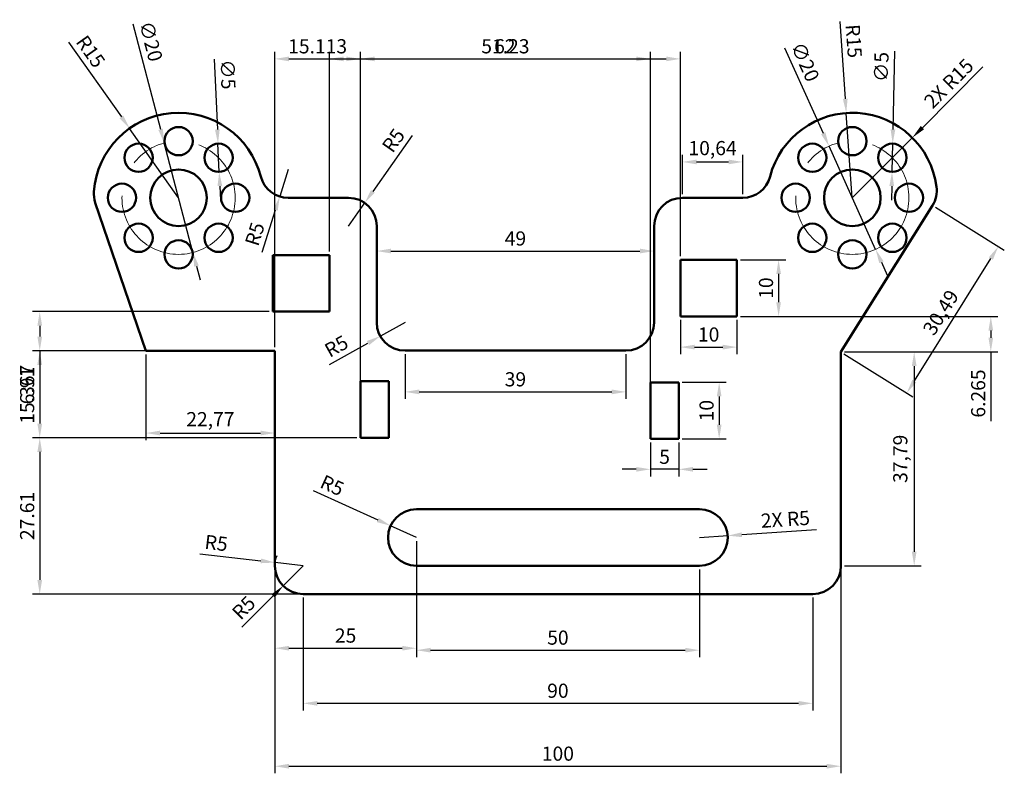
# Model space of a CAD drawing. Units: millimetres. Extents: x 1154 to 1562, y 1225 to 1481.
# Tile 3 of 4: x 1388 to 1562, y 1225 to 1358. Entities that reach past the tile are written whole.
import ezdxf

# ---------------------------------------------------------------- set-up
doc = ezdxf.new("R2010")
doc.units = ezdxf.units.MM
doc.linetypes.add('CENTER', pattern=[50.8, 31.75, -6.35, 6.35, -6.35])
for name, color, linetype, lineweight in [('M-CNTR', 1, 'CENTER', 18), ('M-DIMS', 2, 'Continuous', 25), ('M-OUTL', 7, 'Continuous', 50)]:
    doc.layers.add(name, color=color, linetype=linetype, lineweight=lineweight)
doc.styles.get("Standard").update_dxf_attribs({"font": 'arial.ttf'})
doc.dimstyles.new('ISO-25', dxfattribs={"dimtxt": 2.5, "dimasz": 2.5, "dimexe": 1.25, "dimexo": 0.625, "dimtad": 1, "dimtxsty": 'Standard', "dimcen": 2.5, "dimadec": 0, "dimazin": 0, "dimtfac": 1, "dimtmove": 0, "dimatfit": 3, "dimfxl": 1, "dimarcsym": 0})

# ---------------------------------------------------------------- blocks, each defined once
blk = doc.blocks.new('*U3')
blk.add_circle((0, 0), 2.5)
blk = doc.blocks.new('*U4')
at = {"layer": 'M-OUTL', "color": 0, "linetype": 'ByBlock', "lineweight": -2, "transparency": 16777216}
blk.add_blockref('*U3', (1535.28, 1336.67), dxfattribs=at)
for p, rotation in [((1528.21, 1333.74), 45.00000000000001), ((1542.35, 1333.74), 315), ((1525.28, 1326.67), 90), ((1545.28, 1326.67), 270), ((1528.21, 1319.6), 135), ((1542.35, 1319.6), 225), ((1535.28, 1316.67), 180)]:
    blk.add_blockref('*U3', p, dxfattribs=dict(at, rotation=rotation))
blk = doc.blocks.new('*U5')
blk.add_circle((0, 0), 2.5)
blk = doc.blocks.new('*U6')
at = {"layer": 'M-OUTL', "color": 0, "linetype": 'ByBlock', "lineweight": -2, "transparency": 16777216}
blk.add_blockref('*U5', (1416.28, 1336.67), dxfattribs=at)
for p, rotation in [((1409.21, 1333.74), 45.00000000000001), ((1423.35, 1333.74), 315), ((1406.28, 1326.67), 90), ((1426.28, 1326.67), 270), ((1409.21, 1319.6), 135), ((1423.35, 1319.6), 225), ((1416.28, 1316.67), 180)]:
    blk.add_blockref('*U5', p, dxfattribs=dict(at, rotation=rotation))
blk = doc.blocks.new('*D32')
at = {"layer": 'Defpoints', "color": 0, "transparency": 16777216}
for p in [(1407.63, 1338.92), (1416.28, 1326.67)]:
    blk.add_point(p, dxfattribs=at)
at = {"layer": 'M-DIMS', "color": 0, "lineweight": -2, "transparency": 16777216}
for p, q in [((1396.85, 1354.17), (1406.18, 1340.97)), ((1416.28, 1326.67), (1407.63, 1338.92))]:
    blk.add_line(p, q, dxfattribs=at)
at = {"layer": 'M-DIMS', "color": 0, "transparency": 16777216}
blk.add_solid([(1406.52, 1341.21), (1405.84, 1340.72), (1407.63, 1338.92)], dxfattribs=at)
at = {"layer": 'M-DIMS', "color": 0, "transparency": 16777216, "insert": (1400.49, 1352.31), "char_height": 2.5, "attachment_point": 5, "rotation": 305.247}
blk.add_mtext('R15', dxfattribs=at)
blk = doc.blocks.new('*D33')
at = {"layer": 'Defpoints', "color": 0, "transparency": 16777216}
for p in [(1413.74, 1336.35), (1418.82, 1317)]:
    blk.add_point(p, dxfattribs=at)
at = {"layer": 'M-DIMS', "color": 0, "lineweight": -2, "transparency": 16777216}
for p, q in [((1408.23, 1357.37), (1413.11, 1338.76)), ((1418.82, 1317), (1413.74, 1336.35)), ((1419.45, 1314.58), (1420.09, 1312.16))]:
    blk.add_line(p, q, dxfattribs=at)
at = {"layer": 'M-DIMS', "color": 0, "transparency": 16777216}
for points in [[(1413.51, 1338.87), (1412.71, 1338.66), (1413.74, 1336.35)], [(1419.86, 1314.69), (1419.05, 1314.48), (1418.82, 1317)]]:
    blk.add_solid(points, dxfattribs=at)
at = {"layer": 'M-DIMS', "color": 0, "transparency": 16777216, "insert": (1411.09, 1354.22), "char_height": 2.5, "attachment_point": 5, "rotation": 284.7028}
blk.add_mtext('∅20', dxfattribs=at)
blk = doc.blocks.new('*D34')
at = {"layer": 'Defpoints', "color": 0, "transparency": 16777216}
for p in [(1423.24, 1336.24), (1423.46, 1331.25)]:
    blk.add_point(p, dxfattribs=at)
at = {"layer": 'M-DIMS', "color": 0, "lineweight": -2, "transparency": 16777216}
for p, q in [((1422.58, 1351.16), (1423.13, 1338.74)), ((1423.46, 1331.25), (1423.24, 1336.24)), ((1423.57, 1328.75), (1423.69, 1326.25))]:
    blk.add_line(p, q, dxfattribs=at)
at = {"layer": 'M-DIMS', "color": 0, "transparency": 16777216}
for points in [[(1423.55, 1338.76), (1422.71, 1338.72), (1423.24, 1336.24)], [(1423.99, 1328.77), (1423.16, 1328.73), (1423.46, 1331.25)]]:
    blk.add_solid(points, dxfattribs=at)
at = {"layer": 'M-DIMS', "color": 0, "transparency": 16777216, "insert": (1424.67, 1348.44), "char_height": 2.5, "attachment_point": 5, "rotation": 272.5448}
blk.add_mtext('∅5', dxfattribs=at)
blk = doc.blocks.new('*D35')
at = {"layer": 'Defpoints', "color": 0, "transparency": 16777216}
for p in [(1531.17, 1335.79), (1539.4, 1317.56)]:
    blk.add_point(p, dxfattribs=at)
at = {"layer": 'M-DIMS', "color": 0, "lineweight": -2, "transparency": 16777216}
for p, q in [((1523.32, 1353.17), (1530.14, 1338.07)), ((1539.4, 1317.56), (1531.17, 1335.79)), ((1540.43, 1315.28), (1541.46, 1313))]:
    blk.add_line(p, q, dxfattribs=at)
at = {"layer": 'M-DIMS', "color": 0, "transparency": 16777216}
for points in [[(1530.52, 1338.24), (1529.76, 1337.89), (1531.17, 1335.79)], [(1540.81, 1315.45), (1540.05, 1315.11), (1539.4, 1317.56)]]:
    blk.add_solid(points, dxfattribs=at)
at = {"layer": 'M-DIMS', "color": 0, "transparency": 16777216, "insert": (1526.67, 1350.54), "char_height": 2.5, "attachment_point": 5, "rotation": 294.3018}
blk.add_mtext('∅20', dxfattribs=at)
blk = doc.blocks.new('*D36')
at = {"layer": 'Defpoints', "color": 0, "transparency": 16777216}
for p in [(1542.41, 1336.24), (1542.3, 1331.25)]:
    blk.add_point(p, dxfattribs=at)
at = {"layer": 'M-DIMS', "color": 0, "lineweight": -2, "transparency": 16777216}
for p, q in [((1542.75, 1352.55), (1542.46, 1338.74)), ((1542.3, 1331.25), (1542.41, 1336.24)), ((1542.25, 1328.75), (1542.19, 1326.25))]:
    blk.add_line(p, q, dxfattribs=at)
at = {"layer": 'M-DIMS', "color": 0, "transparency": 16777216}
for points in [[(1542.04, 1338.75), (1542.88, 1338.73), (1542.41, 1336.24)], [(1541.83, 1328.75), (1542.66, 1328.74), (1542.3, 1331.25)]]:
    blk.add_solid(points, dxfattribs=at)
at = {"layer": 'M-DIMS', "color": 0, "transparency": 16777216, "insert": (1540.72, 1349.77), "char_height": 2.5, "attachment_point": 5, "rotation": 88.7888}
blk.add_mtext('∅5', dxfattribs=at)
blk = doc.blocks.new('*D37')
at = {"layer": 'Defpoints', "color": 0, "transparency": 16777216}
for p in [(1534.21, 1341.64), (1535.28, 1326.67)]:
    blk.add_point(p, dxfattribs=at)
at = {"layer": 'M-DIMS', "color": 0, "lineweight": -2, "transparency": 16777216}
for p, q in [((1533.06, 1357.8), (1534.04, 1344.13)), ((1535.28, 1326.67), (1534.21, 1341.64))]:
    blk.add_line(p, q, dxfattribs=at)
at = {"layer": 'M-DIMS', "color": 0, "transparency": 16777216}
blk.add_solid([(1534.45, 1344.16), (1533.62, 1344.1), (1534.21, 1341.64)], dxfattribs=at)
at = {"layer": 'M-DIMS', "color": 0, "transparency": 16777216, "insert": (1535.22, 1354.32), "char_height": 2.5, "attachment_point": 5, "rotation": 274.0804}
blk.add_mtext('R15', dxfattribs=at)
blk = doc.blocks.new('*D38')
at = {"layer": 'Defpoints', "color": 0, "transparency": 16777216}
for p in [(1504.91, 1305.72), (1514.91, 1305.72), (1514.91, 1300.3)]:
    blk.add_point(p, dxfattribs=at)
at = {"layer": 'M-DIMS', "color": 0, "lineweight": -2, "transparency": 16777216}
for p, q in [((1504.91, 1305.1), (1504.91, 1299.05)), ((1514.91, 1305.1), (1514.91, 1299.05)), ((1507.41, 1300.3), (1512.41, 1300.3))]:
    blk.add_line(p, q, dxfattribs=at)
at = {"layer": 'M-DIMS', "color": 0, "transparency": 16777216}
for points in [[(1507.41, 1300.72), (1507.41, 1299.88), (1504.91, 1300.3)], [(1512.41, 1300.72), (1512.41, 1299.88), (1514.91, 1300.3)]]:
    blk.add_solid(points, dxfattribs=at)
at = {"layer": 'M-DIMS', "color": 0, "transparency": 16777216, "insert": (1509.91, 1302.2), "char_height": 2.5, "attachment_point": 5}
blk.add_mtext('10', dxfattribs=at)
blk = doc.blocks.new('*D39')
at = {"layer": 'Defpoints', "color": 0, "transparency": 16777216}
for p in [(1514.91, 1315.72), (1514.91, 1305.72), (1522.26, 1305.72)]:
    blk.add_point(p, dxfattribs=at)
at = {"layer": 'M-DIMS', "color": 0, "lineweight": -2, "transparency": 16777216}
for p, q in [((1515.54, 1315.72), (1523.51, 1315.72)), ((1522.26, 1313.22), (1522.26, 1308.22)), ((1515.54, 1305.72), (1523.51, 1305.72))]:
    blk.add_line(p, q, dxfattribs=at)
at = {"layer": 'M-DIMS', "color": 0, "transparency": 16777216}
for points in [[(1521.85, 1313.22), (1522.68, 1313.22), (1522.26, 1315.72)], [(1521.85, 1308.22), (1522.68, 1308.22), (1522.26, 1305.72)]]:
    blk.add_solid(points, dxfattribs=at)
at = {"layer": 'M-DIMS', "color": 0, "transparency": 16777216, "insert": (1520.36, 1310.72), "char_height": 2.5, "attachment_point": 5, "rotation": 90}
blk.add_mtext('10', dxfattribs=at)
blk = doc.blocks.new('*D40')
at = {"layer": 'Defpoints', "color": 0, "transparency": 16777216}
for p in [(1504.62, 1294.08), (1504.62, 1284.08), (1511.76, 1284.08)]:
    blk.add_point(p, dxfattribs=at)
at = {"layer": 'M-DIMS', "color": 0, "lineweight": -2, "transparency": 16777216}
for p, q in [((1505.25, 1294.08), (1513.01, 1294.08)), ((1511.76, 1291.58), (1511.76, 1286.58)), ((1505.25, 1284.08), (1513.01, 1284.08))]:
    blk.add_line(p, q, dxfattribs=at)
at = {"layer": 'M-DIMS', "color": 0, "transparency": 16777216}
for points in [[(1511.35, 1291.58), (1512.18, 1291.58), (1511.76, 1294.08)], [(1511.35, 1286.58), (1512.18, 1286.58), (1511.76, 1284.08)]]:
    blk.add_solid(points, dxfattribs=at)
at = {"layer": 'M-DIMS', "color": 0, "transparency": 16777216, "insert": (1509.86, 1289.08), "char_height": 2.5, "attachment_point": 5, "rotation": 90}
blk.add_mtext('10', dxfattribs=at)
blk = doc.blocks.new('*D41')
at = {"layer": 'Defpoints', "color": 0, "transparency": 16777216}
for p in [(1499.62, 1284.08), (1504.62, 1284.08), (1499.62, 1278.72)]:
    blk.add_point(p, dxfattribs=at)
at = {"layer": 'M-DIMS', "color": 0, "lineweight": -2, "transparency": 16777216}
for p, q in [((1499.62, 1283.45), (1499.62, 1277.47)), ((1504.62, 1283.45), (1504.62, 1277.47)), ((1497.12, 1278.72), (1494.62, 1278.72)), ((1504.62, 1278.72), (1499.62, 1278.72)), ((1507.12, 1278.72), (1509.62, 1278.72))]:
    blk.add_line(p, q, dxfattribs=at)
at = {"layer": 'M-DIMS', "color": 0, "transparency": 16777216}
for points in [[(1497.12, 1279.13), (1497.12, 1278.3), (1499.62, 1278.72)], [(1507.12, 1279.13), (1507.12, 1278.3), (1504.62, 1278.72)]]:
    blk.add_solid(points, dxfattribs=at)
at = {"layer": 'M-DIMS', "color": 0, "transparency": 16777216, "insert": (1502.12, 1280.61), "char_height": 2.5, "attachment_point": 5}
blk.add_mtext('5', dxfattribs=at)
blk = doc.blocks.new('*D42')
at = {"layer": 'Defpoints', "color": 0, "transparency": 16777216}
for p in [(1458.28, 1261.67), (1508.28, 1261.67), (1508.28, 1246.77)]:
    blk.add_point(p, dxfattribs=at)
at = {"layer": 'M-DIMS', "color": 0, "lineweight": -2, "transparency": 16777216}
for p, q in [((1458.28, 1261.05), (1458.28, 1245.52)), ((1508.28, 1261.05), (1508.28, 1245.52)), ((1460.78, 1246.77), (1505.78, 1246.77))]:
    blk.add_line(p, q, dxfattribs=at)
at = {"layer": 'M-DIMS', "color": 0, "transparency": 16777216}
for points in [[(1460.78, 1247.19), (1460.78, 1246.36), (1458.28, 1246.77)], [(1505.78, 1247.19), (1505.78, 1246.36), (1508.28, 1246.77)]]:
    blk.add_solid(points, dxfattribs=at)
at = {"layer": 'M-DIMS', "color": 0, "transparency": 16777216, "insert": (1483.28, 1248.67), "char_height": 2.5, "attachment_point": 5}
blk.add_mtext('50', dxfattribs=at)
blk = doc.blocks.new('*D43')
at = {"layer": 'Defpoints', "color": 0, "transparency": 16777216}
for p in [(1410.51, 1299.65), (1433.28, 1299.65), (1433.28, 1285.12)]:
    blk.add_point(p, dxfattribs=at)
at = {"layer": 'M-DIMS', "color": 0, "lineweight": -2, "transparency": 16777216}
for p, q in [((1410.51, 1299.02), (1410.51, 1283.87)), ((1433.28, 1299.02), (1433.28, 1283.87)), ((1413.01, 1285.12), (1430.78, 1285.12))]:
    blk.add_line(p, q, dxfattribs=at)
at = {"layer": 'M-DIMS', "color": 0, "transparency": 16777216}
for points in [[(1413.01, 1285.54), (1413.01, 1284.71), (1410.51, 1285.12)], [(1430.78, 1285.54), (1430.78, 1284.71), (1433.28, 1285.12)]]:
    blk.add_solid(points, dxfattribs=at)
at = {"layer": 'M-DIMS', "color": 0, "transparency": 16777216, "insert": (1421.9, 1287.25), "char_height": 2.5, "attachment_point": 5}
blk.add_mtext('22,77', dxfattribs=at)
blk = doc.blocks.new('*D44')
at = {"layer": 'Defpoints', "color": 0, "transparency": 16777216}
for p in [(1453.73, 1268.74), (1458.28, 1266.67)]:
    blk.add_point(p, dxfattribs=at)
at = {"layer": 'M-DIMS', "color": 0, "lineweight": -2, "transparency": 16777216}
for p, q in [((1440.08, 1274.95), (1451.45, 1269.78)), ((1458.28, 1266.67), (1453.73, 1268.74))]:
    blk.add_line(p, q, dxfattribs=at)
at = {"layer": 'M-DIMS', "color": 0, "transparency": 16777216}
blk.add_solid([(1451.63, 1270.16), (1451.28, 1269.4), (1453.73, 1268.74)], dxfattribs=at)
at = {"layer": 'M-DIMS', "color": 0, "transparency": 16777216, "insert": (1443.28, 1275.58), "char_height": 2.5, "attachment_point": 5, "rotation": 335.543}
blk.add_mtext('R5', dxfattribs=at)
blk = doc.blocks.new('*D45')
at = {"layer": 'Defpoints', "color": 0, "transparency": 16777216}
for p in [(1433.32, 1262.25), (1438.28, 1261.67)]:
    blk.add_point(p, dxfattribs=at)
at = {"layer": 'M-DIMS', "color": 0, "lineweight": -2, "transparency": 16777216}
for p, q in [((1420.05, 1263.8), (1430.83, 1262.54)), ((1438.28, 1261.67), (1433.32, 1262.25))]:
    blk.add_line(p, q, dxfattribs=at)
blk.add_arc((1438.28, 1261.67), 5, 159.0215, 180, dxfattribs=at)
at = {"layer": 'M-DIMS', "color": 0, "transparency": 16777216}
blk.add_solid([(1430.88, 1262.96), (1430.78, 1262.13), (1433.32, 1262.25)], dxfattribs=at)
at = {"layer": 'M-DIMS', "color": 0, "transparency": 16777216, "insert": (1422.9, 1265.38), "char_height": 2.5, "attachment_point": 5, "rotation": 353.3454}
blk.add_mtext('R5', dxfattribs=at)
blk = doc.blocks.new('*D46')
at = {"layer": 'Defpoints', "color": 0, "transparency": 16777216}
for p in [(1449.16, 1325.76), (1446.28, 1321.67)]:
    blk.add_point(p, dxfattribs=at)
at = {"layer": 'M-DIMS', "color": 0, "lineweight": -2, "transparency": 16777216}
for p, q in [((1457.56, 1337.69), (1450.6, 1327.8)), ((1446.28, 1321.67), (1449.16, 1325.76))]:
    blk.add_line(p, q, dxfattribs=at)
at = {"layer": 'M-DIMS', "color": 0, "transparency": 16777216}
blk.add_solid([(1450.26, 1328.04), (1450.94, 1327.57), (1449.16, 1325.76)], dxfattribs=at)
at = {"layer": 'M-DIMS', "color": 0, "transparency": 16777216, "insert": (1454.49, 1336.61), "char_height": 2.5, "attachment_point": 5, "rotation": 54.837}
blk.add_mtext('R5', dxfattribs=at)
blk = doc.blocks.new('*D47')
at = {"layer": 'Defpoints', "color": 0, "transparency": 16777216}
for p in [(1435.65, 1331.67), (1434.15, 1326.9)]:
    blk.add_point(p, dxfattribs=at)
at = {"layer": 'M-DIMS', "color": 0, "lineweight": -2, "transparency": 16777216}
for p, q in [((1435.65, 1331.67), (1434.15, 1326.9)), ((1431.07, 1317.07), (1433.41, 1324.52))]:
    blk.add_line(p, q, dxfattribs=at)
at = {"layer": 'M-DIMS', "color": 0, "transparency": 16777216}
blk.add_solid([(1433.01, 1324.64), (1433.8, 1324.39), (1434.15, 1326.9)], dxfattribs=at)
at = {"layer": 'M-DIMS', "color": 0, "transparency": 16777216, "insert": (1430.06, 1320.17), "char_height": 2.5, "attachment_point": 5, "rotation": 72.6131}
blk.add_mtext('R5', dxfattribs=at)
blk = doc.blocks.new('*D48')
at = {"layer": 'Defpoints', "color": 0, "transparency": 16777216}
for p in [(1456.28, 1304.67), (1451.92, 1302.24)]:
    blk.add_point(p, dxfattribs=at)
at = {"layer": 'M-DIMS', "color": 0, "lineweight": -2, "transparency": 16777216}
for p, q in [((1456.28, 1304.67), (1451.92, 1302.24)), ((1442.92, 1297.22), (1449.73, 1301.02))]:
    blk.add_line(p, q, dxfattribs=at)
at = {"layer": 'M-DIMS', "color": 0, "transparency": 16777216}
blk.add_solid([(1449.53, 1301.38), (1449.94, 1300.66), (1451.92, 1302.24)], dxfattribs=at)
at = {"layer": 'M-DIMS', "color": 0, "transparency": 16777216, "insert": (1444.31, 1300.17), "char_height": 2.5, "attachment_point": 5, "rotation": 29.1577}
blk.add_mtext('R5', dxfattribs=at)
blk = doc.blocks.new('*D49')
at = {"layer": 'Defpoints', "color": 0, "transparency": 16777216}
for p in [(1438.28, 1256.67), (1528.28, 1256.67), (1528.28, 1237.39)]:
    blk.add_point(p, dxfattribs=at)
at = {"layer": 'M-DIMS', "color": 0, "lineweight": -2, "transparency": 16777216}
for p, q in [((1438.28, 1256.05), (1438.28, 1236.14)), ((1528.28, 1256.05), (1528.28, 1236.14)), ((1440.78, 1237.39), (1525.78, 1237.39))]:
    blk.add_line(p, q, dxfattribs=at)
at = {"layer": 'M-DIMS', "color": 0, "transparency": 16777216}
for points in [[(1440.78, 1237.8), (1440.78, 1236.97), (1438.28, 1237.39)], [(1525.78, 1237.8), (1525.78, 1236.97), (1528.28, 1237.39)]]:
    blk.add_solid(points, dxfattribs=at)
at = {"layer": 'M-DIMS', "color": 0, "transparency": 16777216, "insert": (1483.28, 1239.29), "char_height": 2.5, "attachment_point": 5}
blk.add_mtext('90', dxfattribs=at)
blk = doc.blocks.new('*D50')
at = {"layer": 'Defpoints', "color": 0, "transparency": 16777216}
for p in [(1433.28, 1261.67), (1533.28, 1261.67), (1533.28, 1226.28)]:
    blk.add_point(p, dxfattribs=at)
at = {"layer": 'M-DIMS', "color": 0, "lineweight": -2, "transparency": 16777216}
for p, q in [((1433.28, 1261.05), (1433.28, 1225.03)), ((1533.28, 1261.05), (1533.28, 1225.03)), ((1435.78, 1226.28), (1530.78, 1226.28))]:
    blk.add_line(p, q, dxfattribs=at)
at = {"layer": 'M-DIMS', "color": 0, "transparency": 16777216}
for points in [[(1435.78, 1226.7), (1435.78, 1225.86), (1433.28, 1226.28)], [(1530.78, 1226.7), (1530.78, 1225.86), (1533.28, 1226.28)]]:
    blk.add_solid(points, dxfattribs=at)
at = {"layer": 'M-DIMS', "color": 0, "transparency": 16777216, "insert": (1483.28, 1228.18), "char_height": 2.5, "attachment_point": 5}
blk.add_mtext('100', dxfattribs=at)
blk = doc.blocks.new('*D59')
at = {"layer": 'Defpoints', "color": 0, "transparency": 16777216}
for p in [(1456.28, 1299.67), (1495.28, 1299.67), (1495.28, 1292.39)]:
    blk.add_point(p, dxfattribs=at)
at = {"layer": 'M-DIMS', "color": 0, "lineweight": -2, "transparency": 16777216}
for p, q in [((1456.28, 1299.05), (1456.28, 1291.14)), ((1495.28, 1299.05), (1495.28, 1291.14)), ((1458.78, 1292.39), (1492.78, 1292.39))]:
    blk.add_line(p, q, dxfattribs=at)
at = {"layer": 'M-DIMS', "color": 0, "transparency": 16777216}
for points in [[(1458.78, 1292.81), (1458.78, 1291.97), (1456.28, 1292.39)], [(1492.78, 1292.81), (1492.78, 1291.97), (1495.28, 1292.39)]]:
    blk.add_solid(points, dxfattribs=at)
at = {"layer": 'M-DIMS', "color": 0, "transparency": 16777216, "insert": (1475.78, 1294.29), "char_height": 2.5, "attachment_point": 5}
blk.add_mtext('39', dxfattribs=at)
blk = doc.blocks.new('*D62')
at = {"layer": 'Defpoints', "color": 0, "transparency": 16777216}
for p in [(1500.28, 1317.26), (1451.28, 1313.17), (1500.28, 1313.17)]:
    blk.add_point(p, dxfattribs=at)
at = {"layer": 'M-DIMS', "color": 0, "lineweight": -2, "transparency": 16777216}
for p, q in [((1451.28, 1313.8), (1451.28, 1318.51)), ((1500.28, 1313.8), (1500.28, 1318.51)), ((1453.78, 1317.26), (1497.78, 1317.26))]:
    blk.add_line(p, q, dxfattribs=at)
at = {"layer": 'M-DIMS', "color": 0, "transparency": 16777216}
for points in [[(1453.78, 1317.68), (1453.78, 1316.85), (1451.28, 1317.26)], [(1497.78, 1317.68), (1497.78, 1316.85), (1500.28, 1317.26)]]:
    blk.add_solid(points, dxfattribs=at)
at = {"layer": 'M-DIMS', "color": 0, "transparency": 16777216, "insert": (1475.78, 1319.16), "char_height": 2.5, "attachment_point": 5}
blk.add_mtext('49', dxfattribs=at)
blk = doc.blocks.new('*D63')
at = {"layer": 'Defpoints', "color": 0, "transparency": 16777216}
for p in [(1515.92, 1333), (1505.28, 1326.67), (1515.92, 1326.67)]:
    blk.add_point(p, dxfattribs=at)
at = {"layer": 'M-DIMS', "color": 0, "lineweight": -2, "transparency": 16777216}
for p, q in [((1505.28, 1327.3), (1505.28, 1334.25)), ((1515.92, 1327.3), (1515.92, 1334.25)), ((1507.78, 1333), (1513.42, 1333))]:
    blk.add_line(p, q, dxfattribs=at)
at = {"layer": 'M-DIMS', "color": 0, "transparency": 16777216}
for points in [[(1507.78, 1333.41), (1507.78, 1332.58), (1505.28, 1333)], [(1513.42, 1333.41), (1513.42, 1332.58), (1515.92, 1333)]]:
    blk.add_solid(points, dxfattribs=at)
at = {"layer": 'M-DIMS', "color": 0, "transparency": 16777216, "insert": (1510.6, 1335.12), "char_height": 2.5, "attachment_point": 5}
blk.add_mtext('10,64', dxfattribs=at)
blk = doc.blocks.new('*D64')
at = {"layer": 'Defpoints', "color": 0, "transparency": 16777216}
for p in [(1549.44, 1325.32), (1561.07, 1318.06), (1533.28, 1299.46)]:
    blk.add_point(p, dxfattribs=at)
at = {"layer": 'M-DIMS', "color": 0, "lineweight": -2, "transparency": 16777216}
for p, q in [((1549.97, 1324.99), (1562.13, 1317.4)), ((1546.24, 1294.32), (1559.74, 1315.94)), ((1533.81, 1299.13), (1545.97, 1291.53))]:
    blk.add_line(p, q, dxfattribs=at)
at = {"layer": 'M-DIMS', "color": 0, "transparency": 16777216}
for points in [[(1559.39, 1316.16), (1560.1, 1315.72), (1561.07, 1318.06)], [(1545.88, 1294.54), (1546.59, 1294.09), (1544.91, 1292.2)]]:
    blk.add_solid(points, dxfattribs=at)
at = {"layer": 'M-DIMS', "color": 0, "transparency": 16777216, "insert": (1551.18, 1306.25), "char_height": 2.5, "attachment_point": 5, "rotation": 58.0079}
blk.add_mtext('30,49', dxfattribs=at)
blk = doc.blocks.new('*D65')
at = {"layer": 'Defpoints', "color": 0, "transparency": 16777216}
for p in [(1533.28, 1299.46), (1533.28, 1261.67), (1546.21, 1261.67)]:
    blk.add_point(p, dxfattribs=at)
at = {"layer": 'M-DIMS', "color": 0, "lineweight": -2, "transparency": 16777216}
for p, q in [((1533.91, 1299.46), (1547.46, 1299.46)), ((1546.21, 1296.96), (1546.21, 1264.17)), ((1533.91, 1261.67), (1547.46, 1261.67))]:
    blk.add_line(p, q, dxfattribs=at)
at = {"layer": 'M-DIMS', "color": 0, "transparency": 16777216}
for points in [[(1545.79, 1296.96), (1546.63, 1296.96), (1546.21, 1299.46)], [(1545.79, 1264.17), (1546.63, 1264.17), (1546.21, 1261.67)]]:
    blk.add_solid(points, dxfattribs=at)
at = {"layer": 'M-DIMS', "color": 0, "transparency": 16777216, "insert": (1544.08, 1280.57), "char_height": 2.5, "attachment_point": 5, "rotation": 90}
blk.add_mtext('37,79', dxfattribs=at)
blk = doc.blocks.new('SLOT-5X10')
for p, q in [((0, 10), (5, 10)), ((0, 0), (0, 10)), ((5, 10), (5, 0)), ((5, 0), (0, 0))]:
    blk.add_line(p, q)
blk = doc.blocks.new('SLOT-10X10')
for p, q in [((0, 10), (10, 10)), ((0, 0), (0, 10)), ((10, 10), (10, 0)), ((10, 0), (0, 0))]:
    blk.add_line(p, q)
blk = doc.blocks.new('*D87')
at = {"layer": 'Defpoints', "color": 0, "transparency": 16777216}
for p in [(1432.92, 1306.56), (1391.76, 1299.65), (1433.28, 1299.65)]:
    blk.add_point(p, dxfattribs=at)
at = {"layer": 'M-DIMS', "color": 0, "lineweight": -2, "transparency": 16777216}
for p, q in [((1432.29, 1306.56), (1390.51, 1306.56)), ((1391.76, 1304.06), (1391.76, 1302.15)), ((1432.66, 1299.65), (1390.51, 1299.65)), ((1391.76, 1299.65), (1391.76, 1289.87))]:
    blk.add_line(p, q, dxfattribs=at)
at = {"layer": 'M-DIMS', "color": 0, "transparency": 16777216}
for points in [[(1391.34, 1304.06), (1392.18, 1304.06), (1391.76, 1306.56)], [(1391.34, 1302.15), (1392.18, 1302.15), (1391.76, 1299.65)]]:
    blk.add_solid(points, dxfattribs=at)
at = {"layer": 'M-DIMS', "color": 0, "transparency": 16777216, "insert": (1389.86, 1293.51), "char_height": 2.5, "attachment_point": 5, "rotation": 90}
blk.add_mtext('6.91', dxfattribs=at)
blk = doc.blocks.new('*D88')
at = {"layer": 'Defpoints', "color": 0, "transparency": 16777216}
for p in [(1433.28, 1299.65), (1391.76, 1284.28), (1448.39, 1284.28)]:
    blk.add_point(p, dxfattribs=at)
at = {"layer": 'M-DIMS', "color": 0, "lineweight": -2, "transparency": 16777216}
for p, q in [((1432.66, 1299.65), (1390.51, 1299.65)), ((1391.76, 1297.15), (1391.76, 1286.78)), ((1447.77, 1284.28), (1390.51, 1284.28))]:
    blk.add_line(p, q, dxfattribs=at)
at = {"layer": 'M-DIMS', "color": 0, "transparency": 16777216}
for points in [[(1391.34, 1297.15), (1392.18, 1297.15), (1391.76, 1299.65)], [(1391.34, 1286.78), (1392.18, 1286.78), (1391.76, 1284.28)]]:
    blk.add_solid(points, dxfattribs=at)
at = {"layer": 'M-DIMS', "color": 0, "transparency": 16777216, "insert": (1389.86, 1291.97), "char_height": 2.5, "attachment_point": 5, "rotation": 90}
blk.add_mtext('15.367', dxfattribs=at)
blk = doc.blocks.new('*D89')
at = {"layer": 'Defpoints', "color": 0, "transparency": 16777216}
for p in [(1448.39, 1284.28), (1391.76, 1256.67), (1438.28, 1256.67)]:
    blk.add_point(p, dxfattribs=at)
at = {"layer": 'M-DIMS', "color": 0, "lineweight": -2, "transparency": 16777216}
for p, q in [((1447.77, 1284.28), (1390.51, 1284.28)), ((1391.76, 1281.78), (1391.76, 1259.17)), ((1437.66, 1256.67), (1390.51, 1256.67))]:
    blk.add_line(p, q, dxfattribs=at)
at = {"layer": 'M-DIMS', "color": 0, "transparency": 16777216}
for points in [[(1391.34, 1281.78), (1392.18, 1281.78), (1391.76, 1284.28)], [(1391.34, 1259.17), (1392.18, 1259.17), (1391.76, 1256.67)]]:
    blk.add_solid(points, dxfattribs=at)
at = {"layer": 'M-DIMS', "color": 0, "transparency": 16777216, "insert": (1389.86, 1270.48), "char_height": 2.5, "attachment_point": 5, "rotation": 90}
blk.add_mtext('27.61', dxfattribs=at)
blk = doc.blocks.new('*D90')
at = {"layer": 'Defpoints', "color": 0, "transparency": 16777216}
for p in [(1504.91, 1351.2), (1442.92, 1316.56), (1504.91, 1315.72)]:
    blk.add_point(p, dxfattribs=at)
at = {"layer": 'M-DIMS', "color": 0, "lineweight": -2, "transparency": 16777216}
for p, q in [((1442.92, 1317.18), (1442.92, 1352.45)), ((1504.91, 1316.35), (1504.91, 1352.45)), ((1445.42, 1351.2), (1502.41, 1351.2))]:
    blk.add_line(p, q, dxfattribs=at)
at = {"layer": 'M-DIMS', "color": 0, "transparency": 16777216}
for points in [[(1445.42, 1351.61), (1445.42, 1350.78), (1442.92, 1351.2)], [(1502.41, 1351.61), (1502.41, 1350.78), (1504.91, 1351.2)]]:
    blk.add_solid(points, dxfattribs=at)
at = {"layer": 'M-DIMS', "color": 0, "transparency": 16777216, "insert": (1473.91, 1353.1), "char_height": 2.5, "attachment_point": 5}
blk.add_mtext('62', dxfattribs=at)
blk = doc.blocks.new('*D91')
at = {"layer": 'Defpoints', "color": 0, "transparency": 16777216}
for p in [(1514.91, 1305.72), (1533.28, 1299.46), (1559.74, 1299.46)]:
    blk.add_point(p, dxfattribs=at)
at = {"layer": 'M-DIMS', "color": 0, "lineweight": -2, "transparency": 16777216}
for p, q in [((1515.54, 1305.72), (1560.99, 1305.72)), ((1559.74, 1303.22), (1559.74, 1301.96)), ((1533.91, 1299.46), (1560.99, 1299.46)), ((1559.74, 1299.46), (1559.74, 1287.24))]:
    blk.add_line(p, q, dxfattribs=at)
at = {"layer": 'M-DIMS', "color": 0, "transparency": 16777216}
for points in [[(1559.33, 1303.22), (1560.16, 1303.22), (1559.74, 1305.72)], [(1559.33, 1301.96), (1560.16, 1301.96), (1559.74, 1299.46)]]:
    blk.add_solid(points, dxfattribs=at)
at = {"layer": 'M-DIMS', "color": 0, "transparency": 16777216, "insert": (1557.84, 1292.1), "char_height": 2.5, "attachment_point": 5, "rotation": 90}
blk.add_mtext('6.265', dxfattribs=at)
blk = doc.blocks.new('*D92')
at = {"layer": 'Defpoints', "color": 0, "transparency": 16777216}
for p in [(1499.62, 1351.2), (1448.39, 1284.28), (1499.62, 1284.08)]:
    blk.add_point(p, dxfattribs=at)
at = {"layer": 'M-DIMS', "color": 0, "lineweight": -2, "transparency": 16777216}
for p, q in [((1448.39, 1284.91), (1448.39, 1352.45)), ((1499.62, 1284.7), (1499.62, 1352.45)), ((1450.89, 1351.2), (1497.12, 1351.2))]:
    blk.add_line(p, q, dxfattribs=at)
at = {"layer": 'M-DIMS', "color": 0, "transparency": 16777216}
for points in [[(1450.89, 1351.61), (1450.89, 1350.78), (1448.39, 1351.2)], [(1497.12, 1351.61), (1497.12, 1350.78), (1499.62, 1351.2)]]:
    blk.add_solid(points, dxfattribs=at)
at = {"layer": 'M-DIMS', "color": 0, "transparency": 16777216, "insert": (1474.01, 1353.1), "char_height": 2.5, "attachment_point": 5}
blk.add_mtext('51.23', dxfattribs=at)
blk = doc.blocks.new('*D93')
at = {"layer": 'Defpoints', "color": 0, "transparency": 16777216}
for p in [(1448.39, 1351.2), (1433.28, 1299.65), (1448.39, 1284.28)]:
    blk.add_point(p, dxfattribs=at)
at = {"layer": 'M-DIMS', "color": 0, "lineweight": -2, "transparency": 16777216}
for p, q in [((1433.28, 1300.27), (1433.28, 1352.45)), ((1448.39, 1284.91), (1448.39, 1352.45)), ((1435.78, 1351.2), (1445.89, 1351.2))]:
    blk.add_line(p, q, dxfattribs=at)
at = {"layer": 'M-DIMS', "color": 0, "transparency": 16777216}
for points in [[(1435.78, 1351.61), (1435.78, 1350.78), (1433.28, 1351.2)], [(1445.89, 1351.61), (1445.89, 1350.78), (1448.39, 1351.2)]]:
    blk.add_solid(points, dxfattribs=at)
at = {"layer": 'M-DIMS', "color": 0, "transparency": 16777216, "insert": (1440.84, 1353.1), "char_height": 2.5, "attachment_point": 5}
blk.add_mtext('15.113', dxfattribs=at)
blk = doc.blocks.new('*D94')
at = {"layer": 'Defpoints', "color": 0, "transparency": 16777216}
for p in [(1458.28, 1266.67), (1433.28, 1261.67), (1458.28, 1247.12)]:
    blk.add_point(p, dxfattribs=at)
at = {"layer": 'M-DIMS', "color": 0, "lineweight": -2, "transparency": 16777216}
for p, q in [((1458.28, 1266.05), (1458.28, 1245.87)), ((1433.28, 1261.05), (1433.28, 1245.87)), ((1435.78, 1247.12), (1455.78, 1247.12))]:
    blk.add_line(p, q, dxfattribs=at)
at = {"layer": 'M-DIMS', "color": 0, "transparency": 16777216}
for points in [[(1435.78, 1247.54), (1435.78, 1246.71), (1433.28, 1247.12)], [(1455.78, 1247.54), (1455.78, 1246.71), (1458.28, 1247.12)]]:
    blk.add_solid(points, dxfattribs=at)
at = {"layer": 'M-DIMS', "color": 0, "transparency": 16777216, "insert": (1445.78, 1249.03), "char_height": 2.5, "attachment_point": 5}
blk.add_mtext('25', dxfattribs=at)
blk = doc.blocks.new('*D101')
at = {"layer": 'Defpoints', "color": 0, "transparency": 16777216}
for p in [(1545.88, 1337.28), (1535.28, 1326.67)]:
    blk.add_point(p, dxfattribs=at)
at = {"layer": 'M-DIMS', "color": 0, "lineweight": -2, "transparency": 16777216}
for p, q in [((1558.36, 1349.77), (1547.65, 1339.05)), ((1535.28, 1326.67), (1545.88, 1337.28))]:
    blk.add_line(p, q, dxfattribs=at)
at = {"layer": 'M-DIMS', "color": 0, "transparency": 16777216}
blk.add_solid([(1547.36, 1339.35), (1547.95, 1338.76), (1545.88, 1337.28)], dxfattribs=at)
at = {"layer": 'M-DIMS', "color": 0, "transparency": 16777216, "insert": (1552.55, 1346.64), "char_height": 2.5, "attachment_point": 5, "rotation": 45.0223}
blk.add_mtext('2X R15', dxfattribs=at)
blk = doc.blocks.new('*D102')
at = {"layer": 'Defpoints', "color": 0, "transparency": 16777216}
for p in [(1508.28, 1266.67), (1513.27, 1267)]:
    blk.add_point(p, dxfattribs=at)
at = {"layer": 'M-DIMS', "color": 0, "lineweight": -2, "transparency": 16777216}
for p, q in [((1528.95, 1268.02), (1515.77, 1267.16)), ((1508.28, 1266.67), (1513.27, 1267))]:
    blk.add_line(p, q, dxfattribs=at)
at = {"layer": 'M-DIMS', "color": 0, "transparency": 16777216}
blk.add_solid([(1515.74, 1267.58), (1515.79, 1266.74), (1513.27, 1267)], dxfattribs=at)
at = {"layer": 'M-DIMS', "color": 0, "transparency": 16777216, "insert": (1523.48, 1269.57), "char_height": 2.5, "attachment_point": 5, "rotation": 3.7216}
blk.add_mtext('2X R5', dxfattribs=at)
blk = doc.blocks.new('*D103')
at = {"layer": 'Defpoints', "color": 0, "transparency": 16777216}
for p in [(1438.28, 1261.67), (1434.75, 1258.13)]:
    blk.add_point(p, dxfattribs=at)
at = {"layer": 'M-DIMS', "color": 0, "lineweight": -2, "transparency": 16777216}
for p, q in [((1438.28, 1261.67), (1434.75, 1258.13)), ((1427.48, 1250.84), (1432.99, 1256.36))]:
    blk.add_line(p, q, dxfattribs=at)
at = {"layer": 'M-DIMS', "color": 0, "transparency": 16777216}
blk.add_solid([(1432.69, 1256.66), (1433.28, 1256.07), (1434.75, 1258.13)], dxfattribs=at)
at = {"layer": 'M-DIMS', "color": 0, "transparency": 16777216, "insert": (1428.01, 1254.05), "char_height": 2.5, "attachment_point": 5, "rotation": 45.0949}
blk.add_mtext('R5', dxfattribs=at)

msp = doc.modelspace()

# ---------------------------------------------------------------- linework, layer by layer
at = {"layer": 'M-CNTR'}
for centre in [(1416.2819, 1326.6736), (1535.2819, 1326.6736)]:
    msp.add_circle(centre, 10, dxfattribs=at)
at = {"layer": 'M-OUTL'}
for p, q in [((1410.5112, 1299.6489), (1401.5782, 1325.8058)), ((1435.6468, 1326.6736), (1446.2819, 1326.6736)), ((1515.9169, 1326.6736), (1505.2819, 1326.6736)), ((1533.2819, 1299.4596), (1549.4379, 1325.3225)), ((1451.2819, 1321.6736), (1451.2819, 1304.6736)), ((1500.2819, 1321.6736), (1500.2819, 1304.6736)), ((1433.2819, 1299.6489), (1410.5112, 1299.6489)), ((1433.2819, 1261.6736), (1433.2819, 1299.6489)), ((1456.2819, 1299.6736), (1495.2819, 1299.6736)), ((1533.2819, 1261.6736), (1533.2819, 1299.4596)), ((1508.2819, 1271.6736), (1458.2819, 1271.6736)), ((1458.2819, 1261.6736), (1508.2819, 1261.6736)), ((1483.2819, 1261.6736), (1458.2819, 1261.6736)), ((1483.2819, 1256.6736), (1438.2819, 1256.6736)), ((1483.2819, 1256.6736), (1528.2819, 1256.6736))]:
    msp.add_line(p, q, dxfattribs=at)
for centre in [(1416.2819, 1326.6736), (1535.2819, 1326.6736)]:
    msp.add_circle(centre, 5, dxfattribs=at)
for centre, radius, start, end in [((1416.2819, 1326.6736), 15, 14.477512, 175.709238), ((1535.2819, 1326.6736), 15, 7.457696, 165.522488), ((1435.6468, 1331.6736), 5, 194.477512, 270), ((1515.9169, 1331.6736), 5, 270, 345.522488), ((1406.3099, 1327.4218), 5, 175.709238, 198.85585), ((1545.1973, 1327.9715), 5, 328.007866, 7.457696), ((1446.2819, 1321.6736), 5, 0, 90), ((1505.2819, 1321.6736), 5, 90, 180), ((1456.2819, 1304.6736), 5, 180, 270), ((1495.2819, 1304.6736), 5, 270, 360), ((1458.2819, 1266.6736), 5, 90, 270), ((1508.2819, 1266.6736), 5, 270, 90), ((1438.2819, 1261.6736), 5, 180, 270), ((1528.2819, 1261.6736), 5, 270, 0)]:
    msp.add_arc(centre, radius, start, end, dxfattribs=at)

# ---------------------------------------------------------------- block references
for name, p in [('*U6', (0, 0)), ('*U4', (0, 0)), ('SLOT-10X10', (1432.915, 1306.559)), ('SLOT-10X10', (1504.9124, 1305.725)), ('SLOT-5X10', (1448.395, 1284.281)), ('SLOT-5X10', (1499.6206, 1284.0771))]:
    msp.add_blockref(name, p, dxfattribs=at)

# ---------------------------------------------------------------- dimensions: what is measured, and where the dimension line sits
at = {"layer": 'M-DIMS'}
for p1, p2, picture, middle in [((1418.8199, 1317.001), (1413.7438, 1336.3461), '*D33', (1409.1841, 1353.7233)), ((1539.3973, 1317.5597), (1531.1664, 1335.7875), '*D35', (1524.8696, 1349.7323)), ((1542.3001, 1331.2452), (1542.4058, 1336.2441), '*D36', (1542.691, 1349.7323)), ((1423.4639, 1331.2471), (1423.2419, 1336.2422), '*D34', (1422.7038, 1348.3509))]:
    dim = msp.add_diameter_dim_2p(p1=p1, p2=p2, dimstyle='ISO-25', override={"dimclrd": 0, "dimclre": 0, "dimclrt": 0}, dxfattribs=at)
    dim.commit()
    dim.dimension.update_dxf_attribs({"geometry": picture, "text_midpoint": middle, "dimtype": 163})
for center, mpoint, picture, middle in [((1535.2819, 1326.6736), (1534.2145, 1341.6356), '*D37', (1533.3194, 1354.1838)), ((1416.2819, 1326.6736), (1407.6253, 1338.9237), '*D32', (1398.9383, 1351.217)), ((1446.2819, 1321.6736), (1449.1614, 1325.7612), '*D46', (1456.0363, 1335.5204)), ((1458.2819, 1266.6736), (1453.7305, 1268.7436), '*D44', (1442.4925, 1273.8549)), ((1438.2819, 1261.6736), (1433.3156, 1262.253), '*D45', (1422.6808, 1263.4938))]:
    dim = msp.add_radius_dim(center=center, mpoint=mpoint, dimstyle='ISO-25', override={"dimclrd": 0, "dimclre": 0, "dimclrt": 0}, dxfattribs=at)
    dim.commit()
    dim.dimension.update_dxf_attribs({"geometry": picture, "text_midpoint": middle, "dimtype": 164})
for base, p1, p2, override, picture, middle in [((1448.3947, 1351.1955), (1433.2819, 1299.6489), (1448.3947, 1284.2814), {"dimdec": 3, "dimlfac": 1, "dimrnd": 0, "dimzin": 0, "dimdsep": 46, "dimlunit": 2}, '*D93', (1440.8383, 1353.0977)), ((1504.9124, 1351.1955), (1442.915, 1316.5588), (1504.9124, 1315.7248), {"dimdec": 0, "dimlfac": 1, "dimrnd": 0, "dimzin": 0, "dimdsep": 46, "dimlunit": 2}, '*D90', (1473.9137, 1353.0969)), ((1499.6203, 1351.1955), (1448.3947, 1284.2814), (1499.6203, 1284.0775), {"dimdec": 2, "dimlfac": 1, "dimrnd": 0, "dimzin": 0, "dimdsep": 46, "dimlunit": 2}, '*D92', (1474.0075, 1353.0977)), ((1515.91695, 1332.99749), (1505.28187, 1326.67359), (1515.91695, 1326.67359), {"dimclrd": 0, "dimclre": 0, "dimclrt": 0}, '*D63', (1510.59941, 1335.12488)), ((1500.2819, 1317.263), (1451.2819, 1313.1736), (1500.2819, 1313.1736), {"dimclrd": 0, "dimclre": 0, "dimclrt": 0}, '*D62', (1475.7819, 1319.1644)), ((1514.9124, 1300.3011), (1504.9124, 1305.7248), (1514.9124, 1305.7248), {"dimclrd": 0, "dimclre": 0, "dimclrt": 0}, '*D38', (1509.9124, 1302.2025)), ((1433.2819, 1285.1235), (1410.5112, 1299.6489), (1433.2819, 1299.6489), {"dimclrd": 0, "dimclre": 0, "dimclrt": 0}, '*D43', (1421.8965, 1287.2509)), ((1495.2819, 1292.3907), (1456.2819, 1299.6736), (1495.2819, 1299.6736), {"dimclrd": 0, "dimclre": 0, "dimclrt": 0}, '*D59', (1475.7819, 1294.293)), ((1499.6203, 1278.716), (1504.6203, 1284.0775), (1499.6203, 1284.0775), {"dimclrd": 0, "dimclre": 0, "dimclrt": 0}, '*D41', (1502.1203, 1280.6123)), ((1458.2819, 1247.1236), (1433.2819, 1261.6736), (1458.2819, 1266.6736), {"dimdec": 0, "dimlfac": 1, "dimrnd": 0, "dimzin": 0, "dimdsep": 46, "dimlunit": 2}, '*D94', (1445.7819, 1249.025)), ((1533.2819, 1226.2809), (1433.2819, 1261.6736), (1533.2819, 1261.6736), {"dimclrd": 0, "dimclre": 0, "dimclrt": 0}, '*D50', (1483.2819, 1228.1823)), ((1508.2819, 1246.7719), (1458.2819, 1261.6736), (1508.2819, 1261.6736), {"dimclrd": 0, "dimclre": 0, "dimclrt": 0}, '*D42', (1483.2819, 1248.6733)), ((1528.2819, 1237.387), (1438.2819, 1256.6736), (1528.2819, 1256.6736), {"dimclrd": 0, "dimclre": 0, "dimclrt": 0}, '*D49', (1483.2819, 1239.2885))]:
    dim = msp.add_linear_dim(base=base, p1=p1, p2=p2, dimstyle='ISO-25', override=override, dxfattribs=at)
    dim.commit()
    dim.dimension.update_dxf_attribs({"geometry": picture, "text_midpoint": middle})
for center, mpoint, picture, middle in [((1535.2819, 1326.6736), (1545.8843, 1337.2843), '*D101', (1552.5466, 1346.6419)), ((1508.2819, 1266.6736), (1513.2713, 1266.9981), '*D102', (1523.4833, 1269.5678))]:
    dim = msp.add_radius_dim(center=center, mpoint=mpoint, text='2X <>', dimstyle='ISO-25', override={"dimdec": 0, "dimlfac": 1, "dimrnd": 0, "dimzin": 0, "dimdsep": 46, "dimlunit": 2}, dxfattribs=at)
    dim.commit()
    dim.dimension.update_dxf_attribs({"geometry": picture, "text_midpoint": middle})
for center, mpoint, override, picture, middle in [((1435.6468, 1331.6736), (1434.1527, 1326.902), {"dimclrd": 0, "dimclre": 0, "dimclrt": 0}, '*D47', (1430.057, 1320.1682)), ((1456.2819, 1304.6736), (1451.9155, 1302.2375), {"dimclrd": 0, "dimclre": 0, "dimclrt": 0}, '*D48', (1444.3109, 1300.1663)), ((1438.2819, 1261.6736), (1434.7522, 1258.1322), {"dimdec": 0, "dimlfac": 1, "dimrnd": 0, "dimzin": 0, "dimdsep": 46, "dimlunit": 2}, '*D103', (1428.0086, 1254.0525))]:
    dim = msp.add_radius_dim(center=center, mpoint=mpoint, dimstyle='ISO-25', override=override, dxfattribs=at)
    dim.commit()
    dim.dimension.update_dxf_attribs({"geometry": picture, "text_midpoint": middle})
dim = msp.add_aligned_dim(p1=(1533.2819, 1299.4596), p2=(1549.4379, 1325.3225), distance=-13.7116, dimstyle='ISO-25', override={"dimclrd": 0, "dimclre": 0, "dimclrt": 0}, dxfattribs=at)
dim.commit()
dim.dimension.update_dxf_attribs({"geometry": '*D64', "text_midpoint": (1551.1847, 1306.2537)})
for base, p1, p2, override, picture, middle in [((1522.2629, 1305.7248), (1514.9124, 1315.7248), (1514.9124, 1305.7248), {"dimclrd": 0, "dimclre": 0, "dimclrt": 0}, '*D39', (1520.3615, 1310.7248)), ((1391.7616, 1299.6489), (1432.915, 1306.5588), (1433.2819, 1299.6489), {"dimdec": 2, "dimlfac": 1, "dimrnd": 0, "dimzin": 0, "dimdsep": 46, "dimlunit": 2}, '*D87', (1389.8602, 1293.5114)), ((1559.7427, 1299.4596), (1514.9124, 1305.7248), (1533.2819, 1299.4596), {"dimdec": 3, "dimlfac": 1, "dimrnd": 0, "dimzin": 0, "dimdsep": 46, "dimlunit": 2}, '*D91', (1557.8413, 1292.1003)), ((1391.76162, 1284.2814), (1433.28187, 1299.64889), (1448.39471, 1284.2814), {"dimdec": 3, "dimlfac": 1, "dimrnd": 0, "dimzin": 0, "dimdsep": 46, "dimlunit": 2}, '*D88', (1389.85933, 1291.96514)), ((1546.2095, 1261.6736), (1533.2819, 1299.4596), (1533.2819, 1261.6736), {"dimclrd": 0, "dimclre": 0, "dimclrt": 0}, '*D65', (1544.0822, 1280.5666)), ((1511.7621, 1284.0775), (1504.6203, 1294.0775), (1504.6203, 1284.0775), {"dimclrd": 0, "dimclre": 0, "dimclrt": 0}, '*D40', (1509.8607, 1289.0775)), ((1391.7616, 1256.6736), (1448.3947, 1284.2814), (1438.2819, 1256.6736), {"dimdec": 2, "dimlfac": 1, "dimrnd": 0, "dimzin": 0, "dimdsep": 46, "dimlunit": 2}, '*D89', (1389.8602, 1270.4775))]:
    dim = msp.add_linear_dim(base=base, p1=p1, p2=p2, angle=90, dimstyle='ISO-25', override=override, dxfattribs=at)
    dim.commit()
    dim.dimension.update_dxf_attribs({"geometry": picture, "text_midpoint": middle})

doc.saveas('drawing.dxf')
